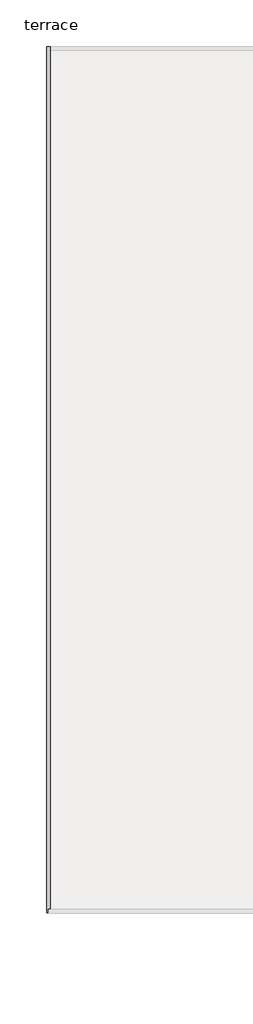
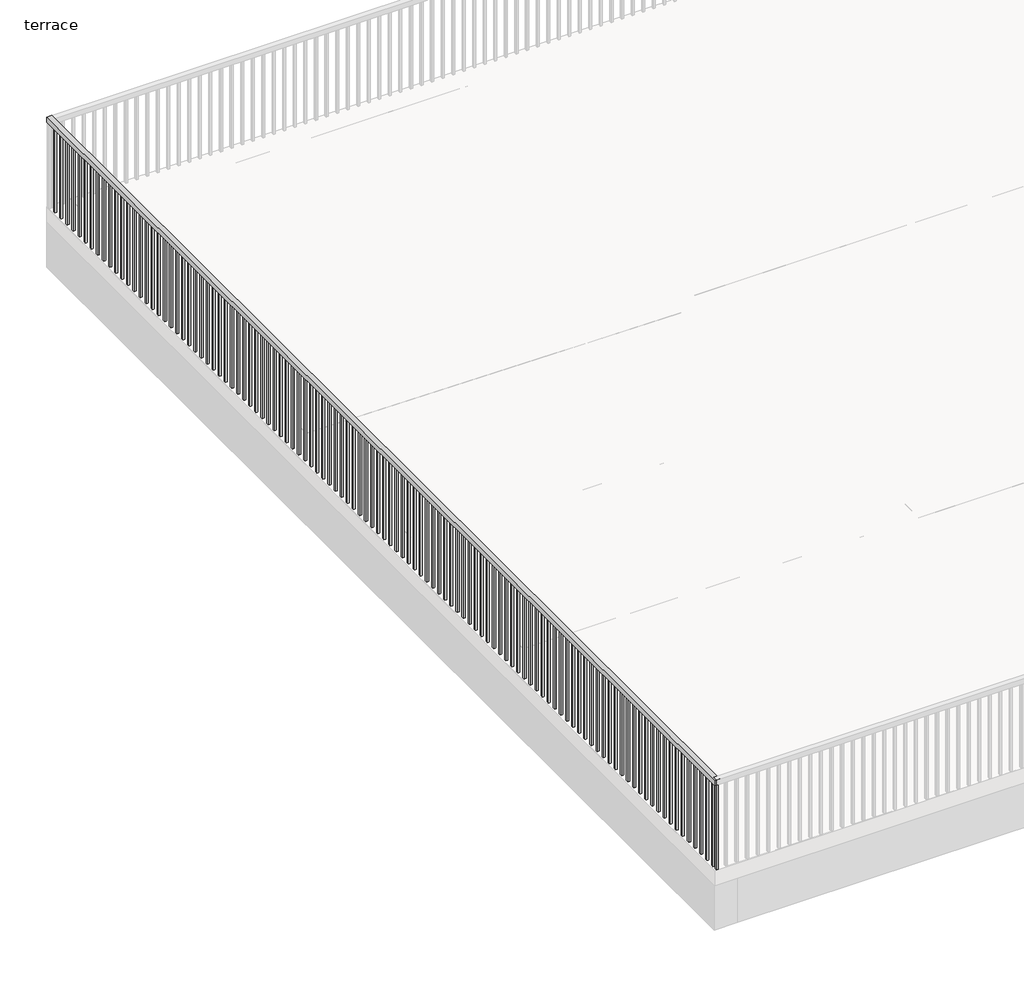
# One storey, part 4 of 6: 1 railing.
"""IFC4 building model written with IfcOpenShell, lengths in millimetres."""

from ifc_helpers import new_model, si_unit, frame, origin, place, context, project, spatial, polyline, outline, extrude, element, save

model = new_model("IFC4")

# Units and contexts
model_context = context("Model", 3, world=origin())
ifc_project = project(units=[si_unit("LENGTHUNIT", "METRE", prefix="MILLI")], contexts=[model_context])

# Site, building, storey
site = spatial("IfcSite", under=ifc_project)
building = spatial("IfcBuilding", under=site)
storey = spatial("IfcBuildingStorey", under=building, Name="terrace", Elevation=7010.4)

# Railing
placement = place(None, origin())
element("IfcRailing", 1, ObjectType="Handrail - Rectangular", at=placement, inside=storey, context=model_context, shape_type="SweptSolid", body=[
    extrude(outline(polyline([(-16300.5993763, 6526.2435985), (-16249.7993763, 6526.2435985), (-16249.7993763, -4611.6564015), (-16300.5993763, -4611.6564015), (-16300.5993763, 6526.2435985)])), frame((0.0, 0.0, 7874.0), z_axis=(0.0, 0.0, 1.0), x_axis=(1.0, 0.0, 0.0)), (0.0, 0.0, 1.0), 50.8),
    extrude(outline(polyline([(-16284.7243763, -4538.6314015), (-16265.6743763, -4538.6314015), (-16265.6743763, -4557.6814015), (-16284.7243763, -4557.6814015), (-16284.7243763, -4538.6314015)])), frame((0.0, 0.0, 7010.4), z_axis=(0.0, 0.0, 1.0), x_axis=(1.0, 0.0, 0.0)), (0.0, 0.0, 1.0), 863.6),
    extrude(outline(polyline([(-16284.7243763, -4437.0314015), (-16265.6743763, -4437.0314015), (-16265.6743763, -4456.0814015), (-16284.7243763, -4456.0814015), (-16284.7243763, -4437.0314015)])), frame((0.0, 0.0, 7010.4), z_axis=(0.0, 0.0, 1.0), x_axis=(1.0, 0.0, 0.0)), (0.0, 0.0, 1.0), 863.6),
    extrude(outline(polyline([(-16284.7243763, -4335.4314015), (-16265.6743763, -4335.4314015), (-16265.6743763, -4354.4814015), (-16284.7243763, -4354.4814015), (-16284.7243763, -4335.4314015)])), frame((0.0, 0.0, 7010.4), z_axis=(0.0, 0.0, 1.0), x_axis=(1.0, 0.0, 0.0)), (0.0, 0.0, 1.0), 863.6),
    extrude(outline(polyline([(-16284.7243763, -4233.8314015), (-16265.6743763, -4233.8314015), (-16265.6743763, -4252.8814015), (-16284.7243763, -4252.8814015), (-16284.7243763, -4233.8314015)])), frame((0.0, 0.0, 7010.4), z_axis=(0.0, 0.0, 1.0), x_axis=(1.0, 0.0, 0.0)), (0.0, 0.0, 1.0), 863.6),
    extrude(outline(polyline([(-16284.7243763, -4132.2314015), (-16265.6743763, -4132.2314015), (-16265.6743763, -4151.2814015), (-16284.7243763, -4151.2814015), (-16284.7243763, -4132.2314015)])), frame((0.0, 0.0, 7010.4), z_axis=(0.0, 0.0, 1.0), x_axis=(1.0, 0.0, 0.0)), (0.0, 0.0, 1.0), 863.6),
    extrude(outline(polyline([(-16284.7243763, -4030.6314015), (-16265.6743763, -4030.6314015), (-16265.6743763, -4049.6814015), (-16284.7243763, -4049.6814015), (-16284.7243763, -4030.6314015)])), frame((0.0, 0.0, 7010.4), z_axis=(0.0, 0.0, 1.0), x_axis=(1.0, 0.0, 0.0)), (0.0, 0.0, 1.0), 863.6),
    extrude(outline(polyline([(-16284.7243763, -3929.0314015), (-16265.6743763, -3929.0314015), (-16265.6743763, -3948.0814015), (-16284.7243763, -3948.0814015), (-16284.7243763, -3929.0314015)])), frame((0.0, 0.0, 7010.4), z_axis=(0.0, 0.0, 1.0), x_axis=(1.0, 0.0, 0.0)), (0.0, 0.0, 1.0), 863.6),
    extrude(outline(polyline([(-16284.7243763, -3827.4314015), (-16265.6743763, -3827.4314015), (-16265.6743763, -3846.4814015), (-16284.7243763, -3846.4814015), (-16284.7243763, -3827.4314015)])), frame((0.0, 0.0, 7010.4), z_axis=(0.0, 0.0, 1.0), x_axis=(1.0, 0.0, 0.0)), (0.0, 0.0, 1.0), 863.6),
    extrude(outline(polyline([(-16284.7243763, -3725.8314015), (-16265.6743763, -3725.8314015), (-16265.6743763, -3744.8814015), (-16284.7243763, -3744.8814015), (-16284.7243763, -3725.8314015)])), frame((0.0, 0.0, 7010.4), z_axis=(0.0, 0.0, 1.0), x_axis=(1.0, 0.0, 0.0)), (0.0, 0.0, 1.0), 863.6),
    extrude(outline(polyline([(-16284.7243763, -3624.2314015), (-16265.6743763, -3624.2314015), (-16265.6743763, -3643.2814015), (-16284.7243763, -3643.2814015), (-16284.7243763, -3624.2314015)])), frame((0.0, 0.0, 7010.4), z_axis=(0.0, 0.0, 1.0), x_axis=(1.0, 0.0, 0.0)), (0.0, 0.0, 1.0), 863.6),
    extrude(outline(polyline([(-16284.7243763, -3522.6314015), (-16265.6743763, -3522.6314015), (-16265.6743763, -3541.6814015), (-16284.7243763, -3541.6814015), (-16284.7243763, -3522.6314015)])), frame((0.0, 0.0, 7010.4), z_axis=(0.0, 0.0, 1.0), x_axis=(1.0, 0.0, 0.0)), (0.0, 0.0, 1.0), 863.6),
    extrude(outline(polyline([(-16284.7243763, -3421.0314015), (-16265.6743763, -3421.0314015), (-16265.6743763, -3440.0814015), (-16284.7243763, -3440.0814015), (-16284.7243763, -3421.0314015)])), frame((0.0, 0.0, 7010.4), z_axis=(0.0, 0.0, 1.0), x_axis=(1.0, 0.0, 0.0)), (0.0, 0.0, 1.0), 863.6),
    extrude(outline(polyline([(-16284.7243763, -3319.4314015), (-16265.6743763, -3319.4314015), (-16265.6743763, -3338.4814015), (-16284.7243763, -3338.4814015), (-16284.7243763, -3319.4314015)])), frame((0.0, 0.0, 7010.4), z_axis=(0.0, 0.0, 1.0), x_axis=(1.0, 0.0, 0.0)), (0.0, 0.0, 1.0), 863.6),
    extrude(outline(polyline([(-16284.7243763, -3217.8314015), (-16265.6743763, -3217.8314015), (-16265.6743763, -3236.8814015), (-16284.7243763, -3236.8814015), (-16284.7243763, -3217.8314015)])), frame((0.0, 0.0, 7010.4), z_axis=(0.0, 0.0, 1.0), x_axis=(1.0, 0.0, 0.0)), (0.0, 0.0, 1.0), 863.6),
    extrude(outline(polyline([(-16284.7243763, -3116.2314015), (-16265.6743763, -3116.2314015), (-16265.6743763, -3135.2814015), (-16284.7243763, -3135.2814015), (-16284.7243763, -3116.2314015)])), frame((0.0, 0.0, 7010.4), z_axis=(0.0, 0.0, 1.0), x_axis=(1.0, 0.0, 0.0)), (0.0, 0.0, 1.0), 863.6),
    extrude(outline(polyline([(-16284.7243763, -3014.6314015), (-16265.6743763, -3014.6314015), (-16265.6743763, -3033.6814015), (-16284.7243763, -3033.6814015), (-16284.7243763, -3014.6314015)])), frame((0.0, 0.0, 7010.4), z_axis=(0.0, 0.0, 1.0), x_axis=(1.0, 0.0, 0.0)), (0.0, 0.0, 1.0), 863.6),
    extrude(outline(polyline([(-16284.7243763, -2913.0314015), (-16265.6743763, -2913.0314015), (-16265.6743763, -2932.0814015), (-16284.7243763, -2932.0814015), (-16284.7243763, -2913.0314015)])), frame((0.0, 0.0, 7010.4), z_axis=(0.0, 0.0, 1.0), x_axis=(1.0, 0.0, 0.0)), (0.0, 0.0, 1.0), 863.6),
    extrude(outline(polyline([(-16284.7243763, -2811.4314015), (-16265.6743763, -2811.4314015), (-16265.6743763, -2830.4814015), (-16284.7243763, -2830.4814015), (-16284.7243763, -2811.4314015)])), frame((0.0, 0.0, 7010.4), z_axis=(0.0, 0.0, 1.0), x_axis=(1.0, 0.0, 0.0)), (0.0, 0.0, 1.0), 863.6),
    extrude(outline(polyline([(-16284.7243763, -2709.8314015), (-16265.6743763, -2709.8314015), (-16265.6743763, -2728.8814015), (-16284.7243763, -2728.8814015), (-16284.7243763, -2709.8314015)])), frame((0.0, 0.0, 7010.4), z_axis=(0.0, 0.0, 1.0), x_axis=(1.0, 0.0, 0.0)), (0.0, 0.0, 1.0), 863.6),
    extrude(outline(polyline([(-16284.7243763, -2608.2314015), (-16265.6743763, -2608.2314015), (-16265.6743763, -2627.2814015), (-16284.7243763, -2627.2814015), (-16284.7243763, -2608.2314015)])), frame((0.0, 0.0, 7010.4), z_axis=(0.0, 0.0, 1.0), x_axis=(1.0, 0.0, 0.0)), (0.0, 0.0, 1.0), 863.6),
    extrude(outline(polyline([(-16284.7243763, -2506.6314015), (-16265.6743763, -2506.6314015), (-16265.6743763, -2525.6814015), (-16284.7243763, -2525.6814015), (-16284.7243763, -2506.6314015)])), frame((0.0, 0.0, 7010.4), z_axis=(0.0, 0.0, 1.0), x_axis=(1.0, 0.0, 0.0)), (0.0, 0.0, 1.0), 863.6),
    extrude(outline(polyline([(-16284.7243763, -2405.0314015), (-16265.6743763, -2405.0314015), (-16265.6743763, -2424.0814015), (-16284.7243763, -2424.0814015), (-16284.7243763, -2405.0314015)])), frame((0.0, 0.0, 7010.4), z_axis=(0.0, 0.0, 1.0), x_axis=(1.0, 0.0, 0.0)), (0.0, 0.0, 1.0), 863.6),
    extrude(outline(polyline([(-16284.7243763, -2303.4314015), (-16265.6743763, -2303.4314015), (-16265.6743763, -2322.4814015), (-16284.7243763, -2322.4814015), (-16284.7243763, -2303.4314015)])), frame((0.0, 0.0, 7010.4), z_axis=(0.0, 0.0, 1.0), x_axis=(1.0, 0.0, 0.0)), (0.0, 0.0, 1.0), 863.6),
    extrude(outline(polyline([(-16284.7243763, -2201.8314015), (-16265.6743763, -2201.8314015), (-16265.6743763, -2220.8814015), (-16284.7243763, -2220.8814015), (-16284.7243763, -2201.8314015)])), frame((0.0, 0.0, 7010.4), z_axis=(0.0, 0.0, 1.0), x_axis=(1.0, 0.0, 0.0)), (0.0, 0.0, 1.0), 863.6),
    extrude(outline(polyline([(-16284.7243763, -2100.2314015), (-16265.6743763, -2100.2314015), (-16265.6743763, -2119.2814015), (-16284.7243763, -2119.2814015), (-16284.7243763, -2100.2314015)])), frame((0.0, 0.0, 7010.4), z_axis=(0.0, 0.0, 1.0), x_axis=(1.0, 0.0, 0.0)), (0.0, 0.0, 1.0), 863.6),
    extrude(outline(polyline([(-16284.7243763, -1998.6314015), (-16265.6743763, -1998.6314015), (-16265.6743763, -2017.6814015), (-16284.7243763, -2017.6814015), (-16284.7243763, -1998.6314015)])), frame((0.0, 0.0, 7010.4), z_axis=(0.0, 0.0, 1.0), x_axis=(1.0, 0.0, 0.0)), (0.0, 0.0, 1.0), 863.6),
    extrude(outline(polyline([(-16284.7243763, -1897.0314015), (-16265.6743763, -1897.0314015), (-16265.6743763, -1916.0814015), (-16284.7243763, -1916.0814015), (-16284.7243763, -1897.0314015)])), frame((0.0, 0.0, 7010.4), z_axis=(0.0, 0.0, 1.0), x_axis=(1.0, 0.0, 0.0)), (0.0, 0.0, 1.0), 863.6),
    extrude(outline(polyline([(-16284.7243763, -1795.4314015), (-16265.6743763, -1795.4314015), (-16265.6743763, -1814.4814015), (-16284.7243763, -1814.4814015), (-16284.7243763, -1795.4314015)])), frame((0.0, 0.0, 7010.4), z_axis=(0.0, 0.0, 1.0), x_axis=(1.0, 0.0, 0.0)), (0.0, 0.0, 1.0), 863.6),
    extrude(outline(polyline([(-16284.7243763, -1693.8314015), (-16265.6743763, -1693.8314015), (-16265.6743763, -1712.8814015), (-16284.7243763, -1712.8814015), (-16284.7243763, -1693.8314015)])), frame((0.0, 0.0, 7010.4), z_axis=(0.0, 0.0, 1.0), x_axis=(1.0, 0.0, 0.0)), (0.0, 0.0, 1.0), 863.6),
    extrude(outline(polyline([(-16284.7243763, -1592.2314015), (-16265.6743763, -1592.2314015), (-16265.6743763, -1611.2814015), (-16284.7243763, -1611.2814015), (-16284.7243763, -1592.2314015)])), frame((0.0, 0.0, 7010.4), z_axis=(0.0, 0.0, 1.0), x_axis=(1.0, 0.0, 0.0)), (0.0, 0.0, 1.0), 863.6),
    extrude(outline(polyline([(-16284.7243763, -1490.6314015), (-16265.6743763, -1490.6314015), (-16265.6743763, -1509.6814015), (-16284.7243763, -1509.6814015), (-16284.7243763, -1490.6314015)])), frame((0.0, 0.0, 7010.4), z_axis=(0.0, 0.0, 1.0), x_axis=(1.0, 0.0, 0.0)), (0.0, 0.0, 1.0), 863.6),
    extrude(outline(polyline([(-16284.7243763, -1389.0314015), (-16265.6743763, -1389.0314015), (-16265.6743763, -1408.0814015), (-16284.7243763, -1408.0814015), (-16284.7243763, -1389.0314015)])), frame((0.0, 0.0, 7010.4), z_axis=(0.0, 0.0, 1.0), x_axis=(1.0, 0.0, 0.0)), (0.0, 0.0, 1.0), 863.6),
    extrude(outline(polyline([(-16284.7243763, -1287.4314015), (-16265.6743763, -1287.4314015), (-16265.6743763, -1306.4814015), (-16284.7243763, -1306.4814015), (-16284.7243763, -1287.4314015)])), frame((0.0, 0.0, 7010.4), z_axis=(0.0, 0.0, 1.0), x_axis=(1.0, 0.0, 0.0)), (0.0, 0.0, 1.0), 863.6),
    extrude(outline(polyline([(-16284.7243763, -1185.8314015), (-16265.6743763, -1185.8314015), (-16265.6743763, -1204.8814015), (-16284.7243763, -1204.8814015), (-16284.7243763, -1185.8314015)])), frame((0.0, 0.0, 7010.4), z_axis=(0.0, 0.0, 1.0), x_axis=(1.0, 0.0, 0.0)), (0.0, 0.0, 1.0), 863.6),
    extrude(outline(polyline([(-16284.7243763, -1084.2314015), (-16265.6743763, -1084.2314015), (-16265.6743763, -1103.2814015), (-16284.7243763, -1103.2814015), (-16284.7243763, -1084.2314015)])), frame((0.0, 0.0, 7010.4), z_axis=(0.0, 0.0, 1.0), x_axis=(1.0, 0.0, 0.0)), (0.0, 0.0, 1.0), 863.6),
    extrude(outline(polyline([(-16284.7243763, -982.6314015), (-16265.6743763, -982.6314015), (-16265.6743763, -1001.6814015), (-16284.7243763, -1001.6814015), (-16284.7243763, -982.6314015)])), frame((0.0, 0.0, 7010.4), z_axis=(0.0, 0.0, 1.0), x_axis=(1.0, 0.0, 0.0)), (0.0, 0.0, 1.0), 863.6),
    extrude(outline(polyline([(-16284.7243763, -881.0314015), (-16265.6743763, -881.0314015), (-16265.6743763, -900.0814015), (-16284.7243763, -900.0814015), (-16284.7243763, -881.0314015)])), frame((0.0, 0.0, 7010.4), z_axis=(0.0, 0.0, 1.0), x_axis=(1.0, 0.0, 0.0)), (0.0, 0.0, 1.0), 863.6),
    extrude(outline(polyline([(-16284.7243763, -779.4314015), (-16265.6743763, -779.4314015), (-16265.6743763, -798.4814015), (-16284.7243763, -798.4814015), (-16284.7243763, -779.4314015)])), frame((0.0, 0.0, 7010.4), z_axis=(0.0, 0.0, 1.0), x_axis=(1.0, 0.0, 0.0)), (0.0, 0.0, 1.0), 863.6),
    extrude(outline(polyline([(-16284.7243763, -677.8314015), (-16265.6743763, -677.8314015), (-16265.6743763, -696.8814015), (-16284.7243763, -696.8814015), (-16284.7243763, -677.8314015)])), frame((0.0, 0.0, 7010.4), z_axis=(0.0, 0.0, 1.0), x_axis=(1.0, 0.0, 0.0)), (0.0, 0.0, 1.0), 863.6),
    extrude(outline(polyline([(-16284.7243763, -576.2314015), (-16265.6743763, -576.2314015), (-16265.6743763, -595.2814015), (-16284.7243763, -595.2814015), (-16284.7243763, -576.2314015)])), frame((0.0, 0.0, 7010.4), z_axis=(0.0, 0.0, 1.0), x_axis=(1.0, 0.0, 0.0)), (0.0, 0.0, 1.0), 863.6),
    extrude(outline(polyline([(-16284.7243763, -474.6314015), (-16265.6743763, -474.6314015), (-16265.6743763, -493.6814015), (-16284.7243763, -493.6814015), (-16284.7243763, -474.6314015)])), frame((0.0, 0.0, 7010.4), z_axis=(0.0, 0.0, 1.0), x_axis=(1.0, 0.0, 0.0)), (0.0, 0.0, 1.0), 863.6),
    extrude(outline(polyline([(-16284.7243763, -373.0314015), (-16265.6743763, -373.0314015), (-16265.6743763, -392.0814015), (-16284.7243763, -392.0814015), (-16284.7243763, -373.0314015)])), frame((0.0, 0.0, 7010.4), z_axis=(0.0, 0.0, 1.0), x_axis=(1.0, 0.0, 0.0)), (0.0, 0.0, 1.0), 863.6),
    extrude(outline(polyline([(-16284.7243763, -271.4314015), (-16265.6743763, -271.4314015), (-16265.6743763, -290.4814015), (-16284.7243763, -290.4814015), (-16284.7243763, -271.4314015)])), frame((0.0, 0.0, 7010.4), z_axis=(0.0, 0.0, 1.0), x_axis=(1.0, 0.0, 0.0)), (0.0, 0.0, 1.0), 863.6),
    extrude(outline(polyline([(-16284.7243763, -169.8314015), (-16265.6743763, -169.8314015), (-16265.6743763, -188.8814015), (-16284.7243763, -188.8814015), (-16284.7243763, -169.8314015)])), frame((0.0, 0.0, 7010.4), z_axis=(0.0, 0.0, 1.0), x_axis=(1.0, 0.0, 0.0)), (0.0, 0.0, 1.0), 863.6),
    extrude(outline(polyline([(-16284.7243763, -68.2314015), (-16265.6743763, -68.2314015), (-16265.6743763, -87.2814015), (-16284.7243763, -87.2814015), (-16284.7243763, -68.2314015)])), frame((0.0, 0.0, 7010.4), z_axis=(0.0, 0.0, 1.0), x_axis=(1.0, 0.0, 0.0)), (0.0, 0.0, 1.0), 863.6),
    extrude(outline(polyline([(-16284.7243763, 33.3685985), (-16265.6743763, 33.3685985), (-16265.6743763, 14.3185985), (-16284.7243763, 14.3185985), (-16284.7243763, 33.3685985)])), frame((0.0, 0.0, 7010.4), z_axis=(0.0, 0.0, 1.0), x_axis=(1.0, 0.0, 0.0)), (0.0, 0.0, 1.0), 863.6),
    extrude(outline(polyline([(-16284.7243763, 134.9685985), (-16265.6743763, 134.9685985), (-16265.6743763, 115.9185985), (-16284.7243763, 115.9185985), (-16284.7243763, 134.9685985)])), frame((0.0, 0.0, 7010.4), z_axis=(0.0, 0.0, 1.0), x_axis=(1.0, 0.0, 0.0)), (0.0, 0.0, 1.0), 863.6),
    extrude(outline(polyline([(-16284.7243763, 236.5685985), (-16265.6743763, 236.5685985), (-16265.6743763, 217.5185985), (-16284.7243763, 217.5185985), (-16284.7243763, 236.5685985)])), frame((0.0, 0.0, 7010.4), z_axis=(0.0, 0.0, 1.0), x_axis=(1.0, 0.0, 0.0)), (0.0, 0.0, 1.0), 863.6),
    extrude(outline(polyline([(-16284.7243763, 338.1685985), (-16265.6743763, 338.1685985), (-16265.6743763, 319.1185985), (-16284.7243763, 319.1185985), (-16284.7243763, 338.1685985)])), frame((0.0, 0.0, 7010.4), z_axis=(0.0, 0.0, 1.0), x_axis=(1.0, 0.0, 0.0)), (0.0, 0.0, 1.0), 863.6),
    extrude(outline(polyline([(-16284.7243763, 439.7685985), (-16265.6743763, 439.7685985), (-16265.6743763, 420.7185985), (-16284.7243763, 420.7185985), (-16284.7243763, 439.7685985)])), frame((0.0, 0.0, 7010.4), z_axis=(0.0, 0.0, 1.0), x_axis=(1.0, 0.0, 0.0)), (0.0, 0.0, 1.0), 863.6),
    extrude(outline(polyline([(-16284.7243763, 541.3685985), (-16265.6743763, 541.3685985), (-16265.6743763, 522.3185985), (-16284.7243763, 522.3185985), (-16284.7243763, 541.3685985)])), frame((0.0, 0.0, 7010.4), z_axis=(0.0, 0.0, 1.0), x_axis=(1.0, 0.0, 0.0)), (0.0, 0.0, 1.0), 863.6),
    extrude(outline(polyline([(-16284.7243763, 642.9685985), (-16265.6743763, 642.9685985), (-16265.6743763, 623.9185985), (-16284.7243763, 623.9185985), (-16284.7243763, 642.9685985)])), frame((0.0, 0.0, 7010.4), z_axis=(0.0, 0.0, 1.0), x_axis=(1.0, 0.0, 0.0)), (0.0, 0.0, 1.0), 863.6),
    extrude(outline(polyline([(-16284.7243763, 744.5685985), (-16265.6743763, 744.5685985), (-16265.6743763, 725.5185985), (-16284.7243763, 725.5185985), (-16284.7243763, 744.5685985)])), frame((0.0, 0.0, 7010.4), z_axis=(0.0, 0.0, 1.0), x_axis=(1.0, 0.0, 0.0)), (0.0, 0.0, 1.0), 863.6),
    extrude(outline(polyline([(-16284.7243763, 846.1685985), (-16265.6743763, 846.1685985), (-16265.6743763, 827.1185985), (-16284.7243763, 827.1185985), (-16284.7243763, 846.1685985)])), frame((0.0, 0.0, 7010.4), z_axis=(0.0, 0.0, 1.0), x_axis=(1.0, 0.0, 0.0)), (0.0, 0.0, 1.0), 863.6),
    extrude(outline(polyline([(-16284.7243763, 947.7685985), (-16265.6743763, 947.7685985), (-16265.6743763, 928.7185985), (-16284.7243763, 928.7185985), (-16284.7243763, 947.7685985)])), frame((0.0, 0.0, 7010.4), z_axis=(0.0, 0.0, 1.0), x_axis=(1.0, 0.0, 0.0)), (0.0, 0.0, 1.0), 863.6),
    extrude(outline(polyline([(-16284.7243763, 1049.3685985), (-16265.6743763, 1049.3685985), (-16265.6743763, 1030.3185985), (-16284.7243763, 1030.3185985), (-16284.7243763, 1049.3685985)])), frame((0.0, 0.0, 7010.4), z_axis=(0.0, 0.0, 1.0), x_axis=(1.0, 0.0, 0.0)), (0.0, 0.0, 1.0), 863.6),
    extrude(outline(polyline([(-16284.7243763, 1150.9685985), (-16265.6743763, 1150.9685985), (-16265.6743763, 1131.9185985), (-16284.7243763, 1131.9185985), (-16284.7243763, 1150.9685985)])), frame((0.0, 0.0, 7010.4), z_axis=(0.0, 0.0, 1.0), x_axis=(1.0, 0.0, 0.0)), (0.0, 0.0, 1.0), 863.6),
    extrude(outline(polyline([(-16284.7243763, 1252.5685985), (-16265.6743763, 1252.5685985), (-16265.6743763, 1233.5185985), (-16284.7243763, 1233.5185985), (-16284.7243763, 1252.5685985)])), frame((0.0, 0.0, 7010.4), z_axis=(0.0, 0.0, 1.0), x_axis=(1.0, 0.0, 0.0)), (0.0, 0.0, 1.0), 863.6),
    extrude(outline(polyline([(-16284.7243763, 1354.1685985), (-16265.6743763, 1354.1685985), (-16265.6743763, 1335.1185985), (-16284.7243763, 1335.1185985), (-16284.7243763, 1354.1685985)])), frame((0.0, 0.0, 7010.4), z_axis=(0.0, 0.0, 1.0), x_axis=(1.0, 0.0, 0.0)), (0.0, 0.0, 1.0), 863.6),
    extrude(outline(polyline([(-16284.7243763, 1455.7685985), (-16265.6743763, 1455.7685985), (-16265.6743763, 1436.7185985), (-16284.7243763, 1436.7185985), (-16284.7243763, 1455.7685985)])), frame((0.0, 0.0, 7010.4), z_axis=(0.0, 0.0, 1.0), x_axis=(1.0, 0.0, 0.0)), (0.0, 0.0, 1.0), 863.6),
    extrude(outline(polyline([(-16284.7243763, 1557.3685985), (-16265.6743763, 1557.3685985), (-16265.6743763, 1538.3185985), (-16284.7243763, 1538.3185985), (-16284.7243763, 1557.3685985)])), frame((0.0, 0.0, 7010.4), z_axis=(0.0, 0.0, 1.0), x_axis=(1.0, 0.0, 0.0)), (0.0, 0.0, 1.0), 863.6),
    extrude(outline(polyline([(-16284.7243763, 1658.9685985), (-16265.6743763, 1658.9685985), (-16265.6743763, 1639.9185985), (-16284.7243763, 1639.9185985), (-16284.7243763, 1658.9685985)])), frame((0.0, 0.0, 7010.4), z_axis=(0.0, 0.0, 1.0), x_axis=(1.0, 0.0, 0.0)), (0.0, 0.0, 1.0), 863.6),
    extrude(outline(polyline([(-16284.7243763, 1760.5685985), (-16265.6743763, 1760.5685985), (-16265.6743763, 1741.5185985), (-16284.7243763, 1741.5185985), (-16284.7243763, 1760.5685985)])), frame((0.0, 0.0, 7010.4), z_axis=(0.0, 0.0, 1.0), x_axis=(1.0, 0.0, 0.0)), (0.0, 0.0, 1.0), 863.6),
    extrude(outline(polyline([(-16284.7243763, 1862.1685985), (-16265.6743763, 1862.1685985), (-16265.6743763, 1843.1185985), (-16284.7243763, 1843.1185985), (-16284.7243763, 1862.1685985)])), frame((0.0, 0.0, 7010.4), z_axis=(0.0, 0.0, 1.0), x_axis=(1.0, 0.0, 0.0)), (0.0, 0.0, 1.0), 863.6),
    extrude(outline(polyline([(-16284.7243763, 1963.7685985), (-16265.6743763, 1963.7685985), (-16265.6743763, 1944.7185985), (-16284.7243763, 1944.7185985), (-16284.7243763, 1963.7685985)])), frame((0.0, 0.0, 7010.4), z_axis=(0.0, 0.0, 1.0), x_axis=(1.0, 0.0, 0.0)), (0.0, 0.0, 1.0), 863.6),
    extrude(outline(polyline([(-16284.7243763, 2065.3685985), (-16265.6743763, 2065.3685985), (-16265.6743763, 2046.3185985), (-16284.7243763, 2046.3185985), (-16284.7243763, 2065.3685985)])), frame((0.0, 0.0, 7010.4), z_axis=(0.0, 0.0, 1.0), x_axis=(1.0, 0.0, 0.0)), (0.0, 0.0, 1.0), 863.6),
    extrude(outline(polyline([(-16284.7243763, 2166.9685985), (-16265.6743763, 2166.9685985), (-16265.6743763, 2147.9185985), (-16284.7243763, 2147.9185985), (-16284.7243763, 2166.9685985)])), frame((0.0, 0.0, 7010.4), z_axis=(0.0, 0.0, 1.0), x_axis=(1.0, 0.0, 0.0)), (0.0, 0.0, 1.0), 863.6),
    extrude(outline(polyline([(-16284.7243763, 2268.5685985), (-16265.6743763, 2268.5685985), (-16265.6743763, 2249.5185985), (-16284.7243763, 2249.5185985), (-16284.7243763, 2268.5685985)])), frame((0.0, 0.0, 7010.4), z_axis=(0.0, 0.0, 1.0), x_axis=(1.0, 0.0, 0.0)), (0.0, 0.0, 1.0), 863.6),
    extrude(outline(polyline([(-16284.7243763, 2370.1685985), (-16265.6743763, 2370.1685985), (-16265.6743763, 2351.1185985), (-16284.7243763, 2351.1185985), (-16284.7243763, 2370.1685985)])), frame((0.0, 0.0, 7010.4), z_axis=(0.0, 0.0, 1.0), x_axis=(1.0, 0.0, 0.0)), (0.0, 0.0, 1.0), 863.6),
    extrude(outline(polyline([(-16284.7243763, 2471.7685985), (-16265.6743763, 2471.7685985), (-16265.6743763, 2452.7185985), (-16284.7243763, 2452.7185985), (-16284.7243763, 2471.7685985)])), frame((0.0, 0.0, 7010.4), z_axis=(0.0, 0.0, 1.0), x_axis=(1.0, 0.0, 0.0)), (0.0, 0.0, 1.0), 863.6),
    extrude(outline(polyline([(-16284.7243763, 2573.3685985), (-16265.6743763, 2573.3685985), (-16265.6743763, 2554.3185985), (-16284.7243763, 2554.3185985), (-16284.7243763, 2573.3685985)])), frame((0.0, 0.0, 7010.4), z_axis=(0.0, 0.0, 1.0), x_axis=(1.0, 0.0, 0.0)), (0.0, 0.0, 1.0), 863.6),
    extrude(outline(polyline([(-16284.7243763, 2674.9685985), (-16265.6743763, 2674.9685985), (-16265.6743763, 2655.9185985), (-16284.7243763, 2655.9185985), (-16284.7243763, 2674.9685985)])), frame((0.0, 0.0, 7010.4), z_axis=(0.0, 0.0, 1.0), x_axis=(1.0, 0.0, 0.0)), (0.0, 0.0, 1.0), 863.6),
    extrude(outline(polyline([(-16284.7243763, 2776.5685985), (-16265.6743763, 2776.5685985), (-16265.6743763, 2757.5185985), (-16284.7243763, 2757.5185985), (-16284.7243763, 2776.5685985)])), frame((0.0, 0.0, 7010.4), z_axis=(0.0, 0.0, 1.0), x_axis=(1.0, 0.0, 0.0)), (0.0, 0.0, 1.0), 863.6),
    extrude(outline(polyline([(-16284.7243763, 2878.1685985), (-16265.6743763, 2878.1685985), (-16265.6743763, 2859.1185985), (-16284.7243763, 2859.1185985), (-16284.7243763, 2878.1685985)])), frame((0.0, 0.0, 7010.4), z_axis=(0.0, 0.0, 1.0), x_axis=(1.0, 0.0, 0.0)), (0.0, 0.0, 1.0), 863.6),
    extrude(outline(polyline([(-16284.7243763, 2979.7685985), (-16265.6743763, 2979.7685985), (-16265.6743763, 2960.7185985), (-16284.7243763, 2960.7185985), (-16284.7243763, 2979.7685985)])), frame((0.0, 0.0, 7010.4), z_axis=(0.0, 0.0, 1.0), x_axis=(1.0, 0.0, 0.0)), (0.0, 0.0, 1.0), 863.6),
    extrude(outline(polyline([(-16284.7243763, 3081.3685985), (-16265.6743763, 3081.3685985), (-16265.6743763, 3062.3185985), (-16284.7243763, 3062.3185985), (-16284.7243763, 3081.3685985)])), frame((0.0, 0.0, 7010.4), z_axis=(0.0, 0.0, 1.0), x_axis=(1.0, 0.0, 0.0)), (0.0, 0.0, 1.0), 863.6),
    extrude(outline(polyline([(-16284.7243763, 3182.9685985), (-16265.6743763, 3182.9685985), (-16265.6743763, 3163.9185985), (-16284.7243763, 3163.9185985), (-16284.7243763, 3182.9685985)])), frame((0.0, 0.0, 7010.4), z_axis=(0.0, 0.0, 1.0), x_axis=(1.0, 0.0, 0.0)), (0.0, 0.0, 1.0), 863.6),
    extrude(outline(polyline([(-16284.7243763, 3284.5685985), (-16265.6743763, 3284.5685985), (-16265.6743763, 3265.5185985), (-16284.7243763, 3265.5185985), (-16284.7243763, 3284.5685985)])), frame((0.0, 0.0, 7010.4), z_axis=(0.0, 0.0, 1.0), x_axis=(1.0, 0.0, 0.0)), (0.0, 0.0, 1.0), 863.6),
    extrude(outline(polyline([(-16284.7243763, 3386.1685985), (-16265.6743763, 3386.1685985), (-16265.6743763, 3367.1185985), (-16284.7243763, 3367.1185985), (-16284.7243763, 3386.1685985)])), frame((0.0, 0.0, 7010.4), z_axis=(0.0, 0.0, 1.0), x_axis=(1.0, 0.0, 0.0)), (0.0, 0.0, 1.0), 863.6),
    extrude(outline(polyline([(-16284.7243763, 3487.7685985), (-16265.6743763, 3487.7685985), (-16265.6743763, 3468.7185985), (-16284.7243763, 3468.7185985), (-16284.7243763, 3487.7685985)])), frame((0.0, 0.0, 7010.4), z_axis=(0.0, 0.0, 1.0), x_axis=(1.0, 0.0, 0.0)), (0.0, 0.0, 1.0), 863.6),
    extrude(outline(polyline([(-16284.7243763, 3589.3685985), (-16265.6743763, 3589.3685985), (-16265.6743763, 3570.3185985), (-16284.7243763, 3570.3185985), (-16284.7243763, 3589.3685985)])), frame((0.0, 0.0, 7010.4), z_axis=(0.0, 0.0, 1.0), x_axis=(1.0, 0.0, 0.0)), (0.0, 0.0, 1.0), 863.6),
    extrude(outline(polyline([(-16284.7243763, 3690.9685985), (-16265.6743763, 3690.9685985), (-16265.6743763, 3671.9185985), (-16284.7243763, 3671.9185985), (-16284.7243763, 3690.9685985)])), frame((0.0, 0.0, 7010.4), z_axis=(0.0, 0.0, 1.0), x_axis=(1.0, 0.0, 0.0)), (0.0, 0.0, 1.0), 863.6),
    extrude(outline(polyline([(-16284.7243763, 3792.5685985), (-16265.6743763, 3792.5685985), (-16265.6743763, 3773.5185985), (-16284.7243763, 3773.5185985), (-16284.7243763, 3792.5685985)])), frame((0.0, 0.0, 7010.4), z_axis=(0.0, 0.0, 1.0), x_axis=(1.0, 0.0, 0.0)), (0.0, 0.0, 1.0), 863.6),
    extrude(outline(polyline([(-16284.7243763, 3894.1685985), (-16265.6743763, 3894.1685985), (-16265.6743763, 3875.1185985), (-16284.7243763, 3875.1185985), (-16284.7243763, 3894.1685985)])), frame((0.0, 0.0, 7010.4), z_axis=(0.0, 0.0, 1.0), x_axis=(1.0, 0.0, 0.0)), (0.0, 0.0, 1.0), 863.6),
    extrude(outline(polyline([(-16284.7243763, 3995.7685985), (-16265.6743763, 3995.7685985), (-16265.6743763, 3976.7185985), (-16284.7243763, 3976.7185985), (-16284.7243763, 3995.7685985)])), frame((0.0, 0.0, 7010.4), z_axis=(0.0, 0.0, 1.0), x_axis=(1.0, 0.0, 0.0)), (0.0, 0.0, 1.0), 863.6),
    extrude(outline(polyline([(-16284.7243763, 4097.3685985), (-16265.6743763, 4097.3685985), (-16265.6743763, 4078.3185985), (-16284.7243763, 4078.3185985), (-16284.7243763, 4097.3685985)])), frame((0.0, 0.0, 7010.4), z_axis=(0.0, 0.0, 1.0), x_axis=(1.0, 0.0, 0.0)), (0.0, 0.0, 1.0), 863.6),
    extrude(outline(polyline([(-16284.7243763, 4198.9685985), (-16265.6743763, 4198.9685985), (-16265.6743763, 4179.9185985), (-16284.7243763, 4179.9185985), (-16284.7243763, 4198.9685985)])), frame((0.0, 0.0, 7010.4), z_axis=(0.0, 0.0, 1.0), x_axis=(1.0, 0.0, 0.0)), (0.0, 0.0, 1.0), 863.6),
    extrude(outline(polyline([(-16284.7243763, 4300.5685985), (-16265.6743763, 4300.5685985), (-16265.6743763, 4281.5185985), (-16284.7243763, 4281.5185985), (-16284.7243763, 4300.5685985)])), frame((0.0, 0.0, 7010.4), z_axis=(0.0, 0.0, 1.0), x_axis=(1.0, 0.0, 0.0)), (0.0, 0.0, 1.0), 863.6),
    extrude(outline(polyline([(-16284.7243763, 4402.1685985), (-16265.6743763, 4402.1685985), (-16265.6743763, 4383.1185985), (-16284.7243763, 4383.1185985), (-16284.7243763, 4402.1685985)])), frame((0.0, 0.0, 7010.4), z_axis=(0.0, 0.0, 1.0), x_axis=(1.0, 0.0, 0.0)), (0.0, 0.0, 1.0), 863.6),
    extrude(outline(polyline([(-16284.7243763, 4503.7685985), (-16265.6743763, 4503.7685985), (-16265.6743763, 4484.7185985), (-16284.7243763, 4484.7185985), (-16284.7243763, 4503.7685985)])), frame((0.0, 0.0, 7010.4), z_axis=(0.0, 0.0, 1.0), x_axis=(1.0, 0.0, 0.0)), (0.0, 0.0, 1.0), 863.6),
    extrude(outline(polyline([(-16284.7243763, 4605.3685985), (-16265.6743763, 4605.3685985), (-16265.6743763, 4586.3185985), (-16284.7243763, 4586.3185985), (-16284.7243763, 4605.3685985)])), frame((0.0, 0.0, 7010.4), z_axis=(0.0, 0.0, 1.0), x_axis=(1.0, 0.0, 0.0)), (0.0, 0.0, 1.0), 863.6),
    extrude(outline(polyline([(-16284.7243763, 4706.9685985), (-16265.6743763, 4706.9685985), (-16265.6743763, 4687.9185985), (-16284.7243763, 4687.9185985), (-16284.7243763, 4706.9685985)])), frame((0.0, 0.0, 7010.4), z_axis=(0.0, 0.0, 1.0), x_axis=(1.0, 0.0, 0.0)), (0.0, 0.0, 1.0), 863.6),
    extrude(outline(polyline([(-16284.7243763, 4808.5685985), (-16265.6743763, 4808.5685985), (-16265.6743763, 4789.5185985), (-16284.7243763, 4789.5185985), (-16284.7243763, 4808.5685985)])), frame((0.0, 0.0, 7010.4), z_axis=(0.0, 0.0, 1.0), x_axis=(1.0, 0.0, 0.0)), (0.0, 0.0, 1.0), 863.6),
    extrude(outline(polyline([(-16284.7243763, 4910.1685985), (-16265.6743763, 4910.1685985), (-16265.6743763, 4891.1185985), (-16284.7243763, 4891.1185985), (-16284.7243763, 4910.1685985)])), frame((0.0, 0.0, 7010.4), z_axis=(0.0, 0.0, 1.0), x_axis=(1.0, 0.0, 0.0)), (0.0, 0.0, 1.0), 863.6),
    extrude(outline(polyline([(-16284.7243763, 5011.7685985), (-16265.6743763, 5011.7685985), (-16265.6743763, 4992.7185985), (-16284.7243763, 4992.7185985), (-16284.7243763, 5011.7685985)])), frame((0.0, 0.0, 7010.4), z_axis=(0.0, 0.0, 1.0), x_axis=(1.0, 0.0, 0.0)), (0.0, 0.0, 1.0), 863.6),
    extrude(outline(polyline([(-16284.7243763, 5113.3685985), (-16265.6743763, 5113.3685985), (-16265.6743763, 5094.3185985), (-16284.7243763, 5094.3185985), (-16284.7243763, 5113.3685985)])), frame((0.0, 0.0, 7010.4), z_axis=(0.0, 0.0, 1.0), x_axis=(1.0, 0.0, 0.0)), (0.0, 0.0, 1.0), 863.6),
    extrude(outline(polyline([(-16284.7243763, 5214.9685985), (-16265.6743763, 5214.9685985), (-16265.6743763, 5195.9185985), (-16284.7243763, 5195.9185985), (-16284.7243763, 5214.9685985)])), frame((0.0, 0.0, 7010.4), z_axis=(0.0, 0.0, 1.0), x_axis=(1.0, 0.0, 0.0)), (0.0, 0.0, 1.0), 863.6),
    extrude(outline(polyline([(-16284.7243763, 5316.5685985), (-16265.6743763, 5316.5685985), (-16265.6743763, 5297.5185985), (-16284.7243763, 5297.5185985), (-16284.7243763, 5316.5685985)])), frame((0.0, 0.0, 7010.4), z_axis=(0.0, 0.0, 1.0), x_axis=(1.0, 0.0, 0.0)), (0.0, 0.0, 1.0), 863.6),
    extrude(outline(polyline([(-16284.7243763, 5418.1685985), (-16265.6743763, 5418.1685985), (-16265.6743763, 5399.1185985), (-16284.7243763, 5399.1185985), (-16284.7243763, 5418.1685985)])), frame((0.0, 0.0, 7010.4), z_axis=(0.0, 0.0, 1.0), x_axis=(1.0, 0.0, 0.0)), (0.0, 0.0, 1.0), 863.6),
    extrude(outline(polyline([(-16284.7243763, 5519.7685985), (-16265.6743763, 5519.7685985), (-16265.6743763, 5500.7185985), (-16284.7243763, 5500.7185985), (-16284.7243763, 5519.7685985)])), frame((0.0, 0.0, 7010.4), z_axis=(0.0, 0.0, 1.0), x_axis=(1.0, 0.0, 0.0)), (0.0, 0.0, 1.0), 863.6),
    extrude(outline(polyline([(-16284.7243763, 5621.3685985), (-16265.6743763, 5621.3685985), (-16265.6743763, 5602.3185985), (-16284.7243763, 5602.3185985), (-16284.7243763, 5621.3685985)])), frame((0.0, 0.0, 7010.4), z_axis=(0.0, 0.0, 1.0), x_axis=(1.0, 0.0, 0.0)), (0.0, 0.0, 1.0), 863.6),
    extrude(outline(polyline([(-16284.7243763, 5722.9685985), (-16265.6743763, 5722.9685985), (-16265.6743763, 5703.9185985), (-16284.7243763, 5703.9185985), (-16284.7243763, 5722.9685985)])), frame((0.0, 0.0, 7010.4), z_axis=(0.0, 0.0, 1.0), x_axis=(1.0, 0.0, 0.0)), (0.0, 0.0, 1.0), 863.6),
    extrude(outline(polyline([(-16284.7243763, 5824.5685985), (-16265.6743763, 5824.5685985), (-16265.6743763, 5805.5185985), (-16284.7243763, 5805.5185985), (-16284.7243763, 5824.5685985)])), frame((0.0, 0.0, 7010.4), z_axis=(0.0, 0.0, 1.0), x_axis=(1.0, 0.0, 0.0)), (0.0, 0.0, 1.0), 863.6),
    extrude(outline(polyline([(-16284.7243763, 5926.1685985), (-16265.6743763, 5926.1685985), (-16265.6743763, 5907.1185985), (-16284.7243763, 5907.1185985), (-16284.7243763, 5926.1685985)])), frame((0.0, 0.0, 7010.4), z_axis=(0.0, 0.0, 1.0), x_axis=(1.0, 0.0, 0.0)), (0.0, 0.0, 1.0), 863.6),
    extrude(outline(polyline([(-16284.7243763, 6027.7685985), (-16265.6743763, 6027.7685985), (-16265.6743763, 6008.7185985), (-16284.7243763, 6008.7185985), (-16284.7243763, 6027.7685985)])), frame((0.0, 0.0, 7010.4), z_axis=(0.0, 0.0, 1.0), x_axis=(1.0, 0.0, 0.0)), (0.0, 0.0, 1.0), 863.6),
    extrude(outline(polyline([(-16284.7243763, 6129.3685985), (-16265.6743763, 6129.3685985), (-16265.6743763, 6110.3185985), (-16284.7243763, 6110.3185985), (-16284.7243763, 6129.3685985)])), frame((0.0, 0.0, 7010.4), z_axis=(0.0, 0.0, 1.0), x_axis=(1.0, 0.0, 0.0)), (0.0, 0.0, 1.0), 863.6),
    extrude(outline(polyline([(-16284.7243763, 6230.9685985), (-16265.6743763, 6230.9685985), (-16265.6743763, 6211.9185985), (-16284.7243763, 6211.9185985), (-16284.7243763, 6230.9685985)])), frame((0.0, 0.0, 7010.4), z_axis=(0.0, 0.0, 1.0), x_axis=(1.0, 0.0, 0.0)), (0.0, 0.0, 1.0), 863.6),
    extrude(outline(polyline([(-16284.7243763, 6332.5685985), (-16265.6743763, 6332.5685985), (-16265.6743763, 6313.5185985), (-16284.7243763, 6313.5185985), (-16284.7243763, 6332.5685985)])), frame((0.0, 0.0, 7010.4), z_axis=(0.0, 0.0, 1.0), x_axis=(1.0, 0.0, 0.0)), (0.0, 0.0, 1.0), 863.6),
    extrude(outline(polyline([(-16284.7243763, 6434.1685985), (-16265.6743763, 6434.1685985), (-16265.6743763, 6415.1185985), (-16284.7243763, 6415.1185985), (-16284.7243763, 6434.1685985)])), frame((0.0, 0.0, 7010.4), z_axis=(0.0, 0.0, 1.0), x_axis=(1.0, 0.0, 0.0)), (0.0, 0.0, 1.0), 863.6),
    extrude(outline(polyline([(-16284.7243763, -4592.6064015), (-16265.6743763, -4592.6064015), (-16265.6743763, -4611.6564015), (-16284.7243763, -4611.6564015), (-16284.7243763, -4592.6064015)])), frame((0.0, 0.0, 7010.4), z_axis=(0.0, 0.0, 1.0), x_axis=(1.0, 0.0, 0.0)), (0.0, 0.0, 1.0), 863.6),
    extrude(outline(polyline([(-16284.7243763, 6526.2435985), (-16265.6743763, 6526.2435985), (-16265.6743763, 6507.1935985), (-16284.7243763, 6507.1935985), (-16284.7243763, 6526.2435985)])), frame((0.0, 0.0, 7010.4), z_axis=(0.0, 0.0, 1.0), x_axis=(1.0, 0.0, 0.0)), (0.0, 0.0, 1.0), 863.6),
])

save(model, "model.ifc")

# Revit data of these elements
# Type "Handrail - Rectangular"
#   Assembly Code = "C2010400"
#   built-in parameter 1008612 = 0.0416667 (stored number, unit not read)
#   built-in parameter 1008611 = 0.0416667 (stored number, unit not read)
#   built-in parameter 1008609 = 0.333333 (stored number, unit not read)
#   built-in parameter 1008604 = 0.166667 (stored number, unit not read)
#   built-in parameter 1008603 = 0.166667 (stored number, unit not read)
#   Railing Height = 3' - 0"
#   built-in parameter 1008630 = 2
#   built-in parameter 1008610 = 2
#   built-in parameter 1008618 = Baluster - Square : 3/4"
# Element 1 (IfcRailing, "Handrail - Rectangular")
#   Phase Created = New Construction
